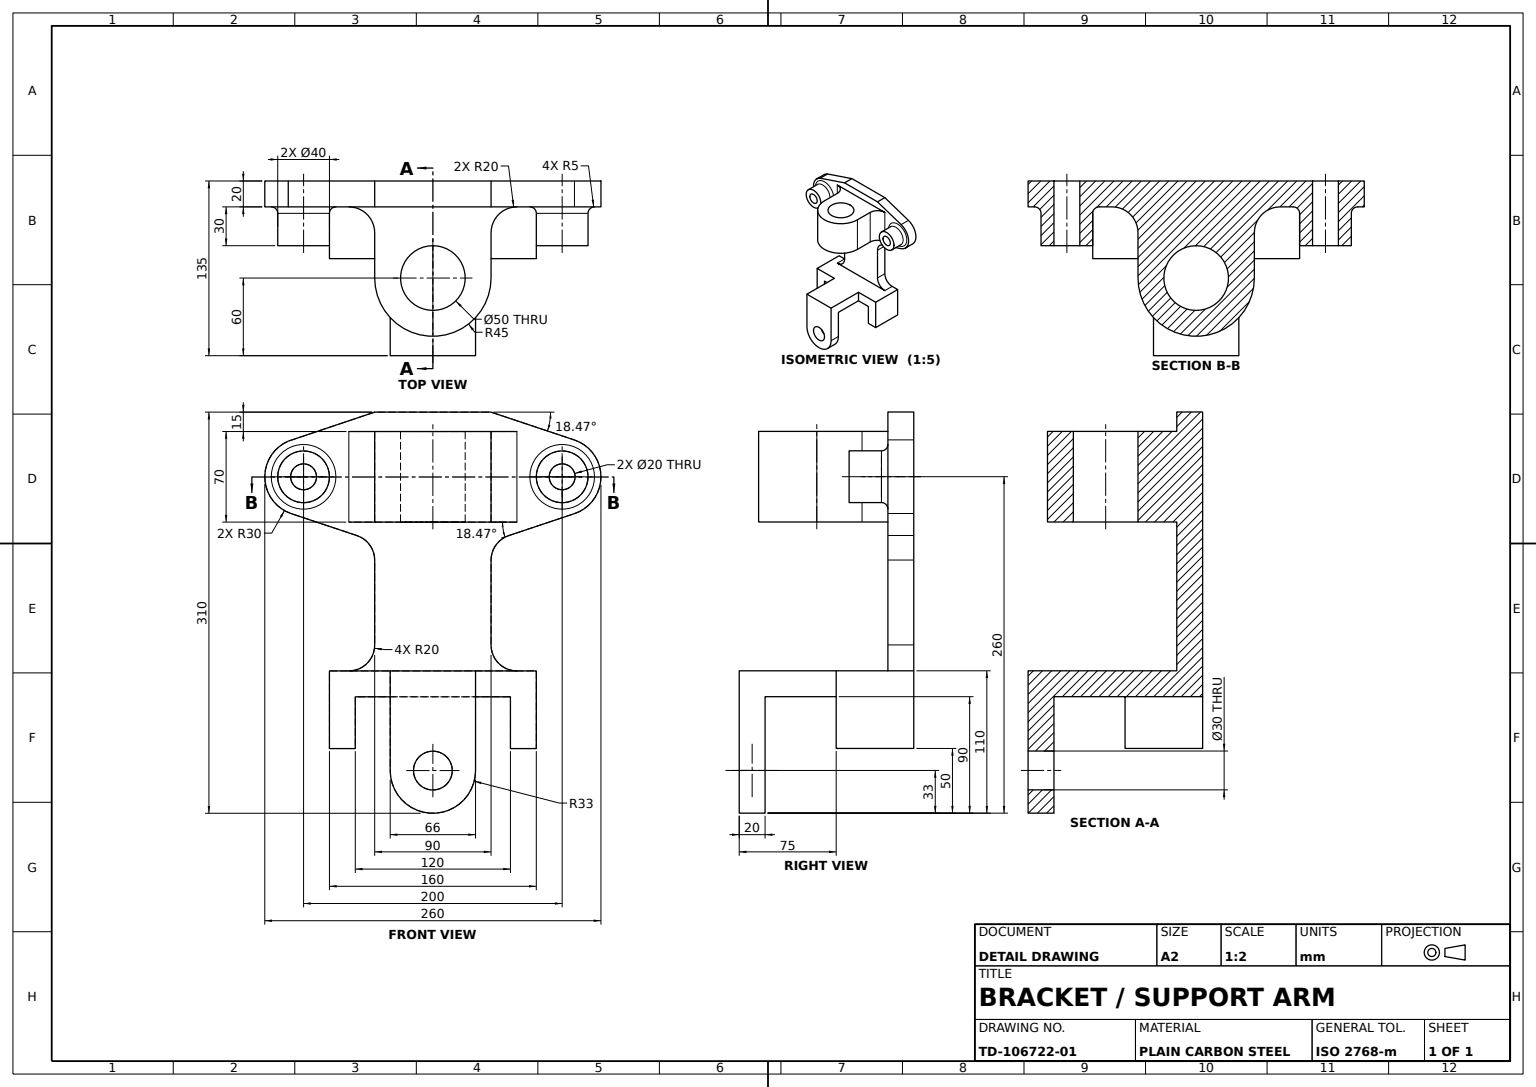
SolidWorks part; units mm, degrees
material "Plain Carbon Steel"
ref_plane "Front Plane" through (0, 0, 0) normal (0, 0, 1) x (1, 0, 0)
ref_plane "Top Plane" through (0, 0, 0) normal (0, 1, 0) x (1, 0, 0)
ref_plane "Right Plane" through (0, 0, 0) normal (1, 0, 0) x (0, 0, -1)
sketch "Base Profile Sketch" plane through (0, 0, 0) normal (0, 0, 1) x (1, 0, 0)
  line L0 (60, 0) -> (80, 0)
  line L1 (80, 0) -> (80, 60)
  line L2 (80, 60) -> (-80, 60)
  line L3 (-80, 60) -> (-80, 0)
  line L4 (-80, 0) -> (-60, 0)
  line L5 (-60, 0) -> (-60, 40)
  line L6 (-60, 40) -> (60, 40)
  line L7 (60, 40) -> (60, 0)
  dimension "D1" = 160
  dimension "D2" = 60
  dimension "D3" = 20
  dimension "D4" = 20
  dimension "D5" = 80
  dimension "D6" = 20
  dimension "D7" = 60
extrude "Base Block" add sketch "Base Profile Sketch" along normal blind 60
sketch "Clevis Lug Sketch" plane through (0, 60, 0) normal (0, 1, 0) x (1, 0, 0)
  line L1 (80, -60) -> (-80, -60) construction
  line L2 (0, -135) -> (33, -135)
  line L3 (33, -135) -> (33, -60)
  line L4 (33, -60) -> (-33, -60)
  line L5 (-33, -60) -> (-33, -135)
  line L6 (-33, -135) -> (0, -135)
  dimension "D1" = 75
  dimension "D2" = 33
  dimension "D3" = 33
  dimension "D4" = 135
extrude "Clevis Lug" add sketch "Clevis Lug Sketch" against normal blind 20
sketch "Lug Extension Sketch" plane through (0, 0, 135) normal (0, 0, 1) x (1, 0, 0)
  line L2 (33, -17) -> (33, 40)
  line L4 (-33, -17) -> (-33, 40)
  line L5 (-33, 40) -> (33, 40)
  arc A0 (-33, -17) -> (33, -17) centre (0, -17) ccw
  dimension "D1" = 17
extrude "Lug Extension" add sketch "Lug Extension Sketch" against normal blind 20
sketch "Pin Hole Sketch Ø30" plane through (0, 0, 135) normal (0, 0, 1) x (1, 0, 0)
  circle A0 centre (0, -17) radius 15
  dimension "D1" = 30
extrude "Clevis Pin Hole Ø30" cut sketch "Pin Hole Sketch Ø30" against normal blind 215
sketch "Upright Web Sketch" plane through (0, 0, 0) normal (0, 0, -1) x (-1, 0, 0)
  line L0 (0, 60) -> (45, 60)
  line L1 (-80, 60) -> (80, 60) construction
  line L2 (45, 60) -> (45, 160)
  line L3 (45, 160) -> (-45, 160)
  line L4 (-45, 160) -> (-45, 60)
  line L5 (-45, 60) -> (0, 60)
  dimension "D1" = 90
  dimension "D2" = 100
  dimension "D3" = 45
extrude "Upright Web" add sketch "Upright Web Sketch" against normal blind 20
sketch "Flange Plate Sketch" plane through (0, 0, 20) normal (0, 0, 1) x (1, 0, 0)
  line L5 (0, 260) -> (45, 260)
  line L6 (45, 260) -> (109.5043, 238.4547)
  line L7 (0, 260) -> (-45, 260)
  line L8 (-45, 260) -> (-111.863, 237.5549)
  line L9 (-109.5043, 181.5453) -> (-45, 160)
  line L10 (109.5043, 181.5453) -> (45, 160)
  line L11 (45, 160) -> (-45, 160)
  arc A0 (109.5043, 181.5453) -> (109.5043, 238.4547) centre (100, 210) ccw
  arc A1 (-111.863, 237.5549) -> (-109.5043, 181.5453) centre (-100, 210) ccw
  dimension "D1" = 30
  dimension "D2" = 30
  dimension "D3" = 200
  dimension "D4" = 210
  dimension "D5" = 100
  dimension "D6" = 100
  dimension "D7" = 64.5043
  dimension "D8" = 90
  dimension "D9" = 66.863
  dimension "D10" = 260
  dimension "D11" = 68.0074
extrude "Flange Plate" add sketch "Flange Plate Sketch" against normal blind 20
fillet "Web-Flange Fillet R20 A" radius 20 1 edges at (-45, 160, 10)
fillet "Web-Flange Fillet R20 B" radius 20 1 edges at (45, 160, 10)
fillet "Web-Base Fillet R20 A" radius 20 1 edges at (45, 60, 10)
fillet "Web-Base Fillet R20 B" radius 20 1 edges at (-45, 60, 10)
ref_plane "Hub Sketch Plane" through (0, 210, 0) normal (0, 1, 0) x (1, 0, 0)
sketch "Hub Sketch" plane through (0, 210, 0) normal (0, 1, 0) x (1, 0, 0)
  line L3 (-45, -75) -> (-45, -20)
  line L4 (-45, -20) -> (45, -20)
  line L5 (45, -20) -> (45, -75)
  arc A0 (-45, -75) -> (45, -75) centre (0, -75) ccw
  dimension "D1" = 75
extrude "Hub Boss" add sketch "Hub Sketch" along normal mid plane 70
fillet "Hub-Web Fillet R20 A" radius 20 1 edges at (-45, 210, 20)
fillet "Hub-Web Fillet R20 B" radius 20 1 edges at (45, 210, 20)
sketch "Mounting Bosses Sketch 2xØ40" plane through (0, 0, 20) normal (0, 0, 1) x (1, 0, 0)
  circle A0 centre (100, 210) radius 20
  circle A1 centre (-100, 210) radius 20
  dimension "D1" = 40
  dimension "D2" = 40
extrude "Mounting Bosses 2xØ40" add sketch "Mounting Bosses Sketch 2xØ40" along normal blind 30
fillet "Mounting Boss Fillet R5 A" radius 5 1 edges at (80, 210, 20)
fillet "Mounting Boss Fillet R5 B" radius 5 1 edges at (-120, 210, 20)
sketch "Hub Bore Sketch Ø50" plane through (0, 245, 0) normal (0, 1, 0) x (1, 0, 0)
  circle A0 centre (0, -75) radius 25
  dimension "D1" = 50
extrude "Hub Bore Ø50" cut sketch "Hub Bore Sketch Ø50" against normal blind 82
sketch "Mounting Holes Sketch 2xØ20" plane through (0, 0, 50) normal (0, 0, 1) x (1, 0, 0)
  circle A0 centre (100, 210) radius 10
  circle A1 centre (-100, 210) radius 10
  dimension "D1" = 20
  dimension "D2" = 20
extrude "Mounting Holes 2xØ20" cut sketch "Mounting Holes Sketch 2xØ20" against normal blind 82
